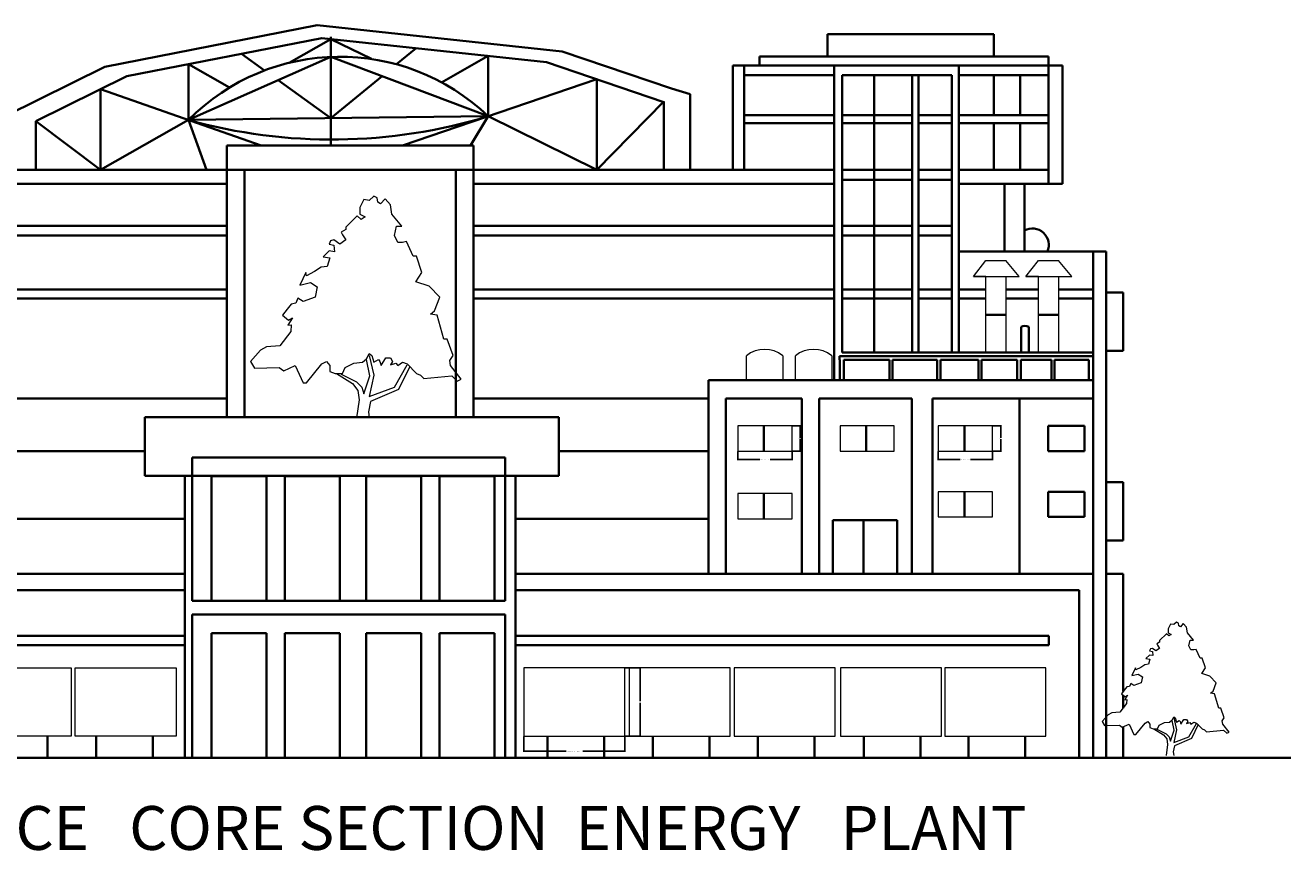
# Model space of a CAD drawing. Units: inches. Extents: x -362 to 223, y -437 to 70.
# Tile 2 of 5: x -124 to 180, y -437 to -239. Entities that reach past the tile are written whole.
import ezdxf

# ---------------------------------------------------------------- set-up
doc = ezdxf.new("R2010")
doc.units = ezdxf.units.IN
doc.header["$MEASUREMENT"] = 0
for name, color, linetype, lineweight in [('A-ANNO-DIMS', 2, 'Continuous', 18), ('A-ANNO-TEXT', 7, 'Continuous', 25), ('A-ELEV', 7, 'Continuous', 35), ('A-EQPM', 8, 'Continuous', 18), ('A-GLAZ', 4, 'Continuous', 18), ('L-PLNT', 3, 'Continuous', 13)]:
    doc.layers.add(name, color=color, linetype=linetype, lineweight=lineweight)
doc.styles.get("Standard").update_dxf_attribs({"font": 'arial.ttf'})
doc.dimstyles.get("Standard").update_dxf_attribs({"dimtxt": 0.18, "dimasz": 0.18, "dimexe": 0.18, "dimexo": 0.0625, "dimgap": 0.09, "dimtad": 0, "dimtih": 1, "dimtoh": 1, "dimdec": 4, "dimzin": 0, "dimdsep": 46, "dimtxsty": 'Standard', "dimcen": 0.09, "dimadec": 0, "dimazin": 0, "dimtfac": 1, "dimtdec": 4, "dimtofl": 0, "dimtmove": 0, "dimatfit": 3, "dimfxl": 1, "dimtolj": 1, "dimtzin": 0, "dimarcsym": 0})

# ---------------------------------------------------------------- blocks, each defined once
blk = doc.blocks.new('*U2')
for points in [[(22.0124, 137.721), (18.5475, 141.5624), (15.5282, 138.2446), (13.8028, 139.3505), (13.3714, 142.1153), (11.2148, 143.2214), (8.1954, 140.4564), (4.7447, 141.0094), (2.1567, 136.0326), (2.1567, 131.6088), (5.6074, 129.9499), (3.0193, 128.2909), (0.4313, 130.5029), (-6.9015, 123.3141), (-6.9015, 121.6552), (-9.9208, 119.9963), (-9.0581, 118.3373), (-6.9015, 115.0195), (-10.7835, 112.2546), (-14.6656, 115.0195), (-16.8222, 114.4665), (-17.6849, 112.2546), (-14.6656, 111.7016), (-14.2342, 107.2778), (-17.6065, 107.8307), (-21.5669, 103.9599), (-17.2536, 103.4069), (-18.9789, 97.8771), (-22.8609, 97.3241), (-27.1743, 94.5593), (-32.3504, 91.7944), (-32.7817, 94.0063), (-36.6638, 85.7116), (-29.7624, 87.3705), (-25.449, 84.6056), (-26.743, 77.9699), (-34.507, 75.205), (-37.9578, 77.4169), (-39.2518, 74.099), (-42.2711, 73.5461), (-44.8592, 70.2282), (-47.8786, 66.3574), (-43.9965, 63.0395), (-41.4085, 64.6985), (-44.3346, 59.8898), (-42.2089, 60.1377), (-42.5159, 55.7849), (-49.6039, 46.4502), (-58.2307, 45.8972), (-62.1127, 43.6853), (-68.5828, 36.4966), (-65.9947, 32.0727), (-50.0352, 32.6257), (-47.0159, 30.4138), (-39.6831, 33.7317), (-34.507, 22.6721), (-32.3504, 22.6721), (-22.4296, 34.8376), (-19.4102, 36.4966), (-17.2536, 33.7317), (-17.2536, 29.8608), (-13.8028, 28.7549), (-9.0581, 28.7549), (-7.3328, 32.6257), (-1.7254, 35.3906), (3.8821, 35.9436), (6.4701, 38.1555), (6.9014, 38.7085), (8.1954, 41.4734), (9.9208, 40.3674), (11.2148, 35.9436), (14.2341, 37.6025), (15.0968, 36.4966), (15.9595, 33.7317), (18.9789, 38.7085), (21.9982, 38.7085), (23.2922, 36.4966), (21.9982, 34.2847), (25.4489, 35.3906), (26.743, 33.7317), (29.7623, 35.9436), (32.7817, 34.8376), (38.8204, 28.7549), (41.4084, 27.6489), (43.5651, 25.437), (61.6813, 27.0959), (65.132, 23.7781), (67.7201, 24.884), (60.8186, 33.7317), (60.3873, 37.0495), (62.544, 40.3674), (58.662, 50.874), (56.5053, 50.874), (52.1919, 66.3574), (47.8785, 66.9103), (50.4665, 69.1222), (53.9172, 77.9699), (47.0158, 85.1586), (38.3891, 87.9235), (42.2711, 94.0063)], [(42.2711, 94.0063), (38.8204, 104.5129), (36.6637, 104.5129), (32.3503, 113.9135), (29.7623, 113.3605), (26.743, 113.3605), (24.5862, 117.7844), (25.8802, 123.8671), (29.331, 123.8671), (22.8609, 131.6088), (21.9982, 137.6916)], [(-9.9208, 28.2019), (0, 23.2251), (3.4507, 19.9072), (4.7447, 15.4834), (8.6267, 27.0959), (6.4701, 37.6025)], [(34.5071, 33.1787), (27.1743, 18.2483), (9.0581, 10.5066), (7.7641, 3.8708), (8.1954, 0)], [(8.1954, 40.3674), (11.2148, 27.6489), (8.1954, 13.8245), (24.5862, 19.9072), (32.7817, 34.2847)], [(-12.9401, 28.7549), (-2.588, 22.1191), (0.8626, 17.6953), (1.7253, 11.6125), (0, 0)]]:
    blk.add_lwpolyline(points)
blk = doc.blocks.new('WIN-STOREFRONT')
for p, q in [((24.23, 16.39), (0, 16.39)), ((0, 16.39), (0, 0)), ((24.23, 0), (24.23, 16.39)), ((0, 0), (6.79, 0)), ((6.79, 0), (24.23, 0))]:
    blk.add_line(p, q)
blk = doc.blocks.new('ROOF-VENT')
for p, q in [((0, 18.24), (2.99, 22.1)), ((2.99, 22.1), (7.83, 22.1)), ((11.03, 18.24), (7.83, 22.1)), ((2.99, 18.24), (0, 18.24)), ((0, 18.24), (11.03, 18.24)), ((2.99, 0), (2.99, 18.24)), ((2.99, 18.24), (7.83, 18.24)), ((7.83, 18.24), (7.83, 0))]:
    blk.add_line(p, q)
blk = doc.blocks.new('WIN-C')
for p, q in [((13.02, 6.07), (0, 6.07)), ((0, 6.07), (0, 5.53)), ((0, 5.53), (0, 0)), ((13.02, 0), (13.02, 6.07)), ((0, 0), (13.02, 0))]:
    blk.add_line(p, q)
blk = doc.blocks.new('WIN-D')
for p, q in [((13.02, 6.07), (0, 6.07)), ((0, 6.07), (0, 5.53)), ((0, 5.53), (0, 0)), ((13.02, 6.07), (11.9, 6.07)), ((13.02, 0), (13.02, 6.07)), ((0, 0), (13.02, 0)), ((11.9, 0), (13.02, 0))]:
    blk.add_line(p, q)
blk = doc.blocks.new('ROOF-DOME')
for p, q in [((0, 0), (0, 5.87)), ((8.74, 5.87), (8.74, 0))]:
    blk.add_line(p, q)
blk.add_arc((4.37, 0.37), 7.03, 51.5309, 128.4691)
blk = doc.blocks.new('*D17')
at = {"layer": 'A-ANNO-DIMS', "color": 0, "lineweight": -2, "transparency": 16777216}
for p, q in [((-4.56, -409.76), (-4.56, -413.51)), ((19.67, -409.76), (19.67, -413.51)), ((-4.38, -413.33), (5.54, -413.33)), ((19.49, -413.33), (9.57, -413.33))]:
    blk.add_line(p, q, dxfattribs=at)
at = {"layer": 'A-ANNO-DIMS', "color": 0, "transparency": 16777216}
for points in [[(-4.38, -413.3), (-4.38, -413.36), (-4.56, -413.33)], [(19.49, -413.3), (19.49, -413.36), (19.67, -413.33)]]:
    blk.add_solid(points, dxfattribs=at)
at = {"layer": 'Defpoints', "color": 0, "transparency": 16777216}
for p in [(-4.56, -409.69), (19.67, -409.69), (19.67, -413.33)]:
    blk.add_point(p, dxfattribs=at)
at = {"layer": 'A-ANNO-DIMS', "color": 0, "transparency": 16777216, "insert": (7.56, -413.33), "char_height": 0.18, "attachment_point": 5}
blk.add_mtext('\\A1;STOREFRONT WINDOW 24 TYP.', dxfattribs=at)
blk = doc.blocks.new('*D18')
at = {"layer": 'A-ANNO-DIMS', "color": 0, "lineweight": -2, "transparency": 16777216}
for p, q in [((19.73, -393.31), (23.48, -393.31)), ((23.3, -393.49), (23.3, -401.32)), ((23.3, -409.51), (23.3, -401.68)), ((19.73, -409.69), (23.48, -409.69))]:
    blk.add_line(p, q, dxfattribs=at)
at = {"layer": 'A-ANNO-DIMS', "color": 0, "transparency": 16777216}
for points in [[(23.27, -393.49), (23.33, -393.49), (23.3, -393.31)], [(23.27, -409.51), (23.33, -409.51), (23.3, -409.69)]]:
    blk.add_solid(points, dxfattribs=at)
at = {"layer": 'Defpoints', "color": 0, "transparency": 16777216}
for p in [(19.67, -393.31), (23.3, -393.31), (19.67, -409.69)]:
    blk.add_point(p, dxfattribs=at)
at = {"layer": 'A-ANNO-DIMS', "color": 0, "transparency": 16777216, "insert": (23.3, -401.5), "char_height": 0.18, "attachment_point": 5}
blk.add_mtext('\\A1;16 TYP.', dxfattribs=at)
blk = doc.blocks.new('*D25')
at = {"layer": 'A-ANNO-DIMS', "color": 0, "lineweight": -2, "transparency": 16777216}
for p, q in [((46.79, -341.37), (46.79, -343.44)), ((46.97, -343.26), (52.05, -343.26)), ((59.62, -343.26), (54.54, -343.26)), ((59.8, -341.37), (59.8, -343.44))]:
    blk.add_line(p, q, dxfattribs=at)
at = {"layer": 'A-ANNO-DIMS', "color": 0, "transparency": 16777216}
for points in [[(46.97, -343.23), (46.97, -343.29), (46.79, -343.26)], [(59.62, -343.23), (59.62, -343.29), (59.8, -343.26)]]:
    blk.add_solid(points, dxfattribs=at)
at = {"layer": 'Defpoints', "color": 0, "transparency": 16777216}
for p in [(46.79, -341.31), (59.8, -341.31), (59.8, -343.26)]:
    blk.add_point(p, dxfattribs=at)
at = {"layer": 'A-ANNO-DIMS', "color": 0, "transparency": 16777216, "insert": (53.29, -343.26), "char_height": 0.18, "attachment_point": 5}
blk.add_mtext('\\A1;WINDOW C 13 TYP.', dxfattribs=at)
blk = doc.blocks.new('*D26')
at = {"layer": 'A-ANNO-DIMS', "color": 0, "lineweight": -2, "transparency": 16777216}
for p, q in [((59.86, -335.24), (61.93, -335.24)), ((61.75, -335.42), (61.75, -338.09)), ((61.75, -341.13), (61.75, -338.45)), ((59.86, -341.31), (61.93, -341.31))]:
    blk.add_line(p, q, dxfattribs=at)
at = {"layer": 'A-ANNO-DIMS', "color": 0, "transparency": 16777216}
for points in [[(61.72, -335.42), (61.78, -335.42), (61.75, -335.24)], [(61.72, -341.13), (61.78, -341.13), (61.75, -341.31)]]:
    blk.add_solid(points, dxfattribs=at)
at = {"layer": 'Defpoints', "color": 0, "transparency": 16777216}
for p in [(59.8, -335.24), (61.75, -335.24), (59.8, -341.31)]:
    blk.add_point(p, dxfattribs=at)
at = {"layer": 'A-ANNO-DIMS', "color": 0, "transparency": 16777216, "insert": (61.75, -338.27), "char_height": 0.18, "attachment_point": 5}
blk.add_mtext('\\A1;6 TYP.', dxfattribs=at)
blk = doc.blocks.new('*D29')
at = {"layer": 'A-ANNO-DIMS', "color": 0, "lineweight": -2, "transparency": 16777216}
for p, q in [((94.91, -341.37), (94.91, -343.44)), ((95.09, -343.26), (100.18, -343.26)), ((107.75, -343.26), (102.66, -343.26)), ((107.93, -341.37), (107.93, -343.44))]:
    blk.add_line(p, q, dxfattribs=at)
at = {"layer": 'A-ANNO-DIMS', "color": 0, "transparency": 16777216}
for points in [[(95.09, -343.23), (95.09, -343.29), (94.91, -343.26)], [(107.75, -343.23), (107.75, -343.29), (107.93, -343.26)]]:
    blk.add_solid(points, dxfattribs=at)
at = {"layer": 'Defpoints', "color": 0, "transparency": 16777216}
for p in [(94.91, -341.31), (107.93, -341.31), (107.93, -343.26)]:
    blk.add_point(p, dxfattribs=at)
at = {"layer": 'A-ANNO-DIMS', "color": 0, "transparency": 16777216, "insert": (101.42, -343.26), "char_height": 0.18, "attachment_point": 5}
blk.add_mtext('\\A1;WINDOW D 13 TYP.', dxfattribs=at)
blk = doc.blocks.new('*D30')
at = {"layer": 'A-ANNO-DIMS', "color": 0, "lineweight": -2, "transparency": 16777216}
for p, q in [((107.99, -335.24), (110.06, -335.24)), ((109.88, -335.42), (109.88, -338.09)), ((109.88, -341.13), (109.88, -338.45)), ((107.99, -341.31), (110.06, -341.31))]:
    blk.add_line(p, q, dxfattribs=at)
at = {"layer": 'A-ANNO-DIMS', "color": 0, "transparency": 16777216}
for points in [[(109.85, -335.42), (109.91, -335.42), (109.88, -335.24)], [(109.85, -341.13), (109.91, -341.13), (109.88, -341.31)]]:
    blk.add_solid(points, dxfattribs=at)
at = {"layer": 'Defpoints', "color": 0, "transparency": 16777216}
for p in [(107.93, -335.24), (109.88, -335.24), (107.93, -341.31)]:
    blk.add_point(p, dxfattribs=at)
at = {"layer": 'A-ANNO-DIMS', "color": 0, "transparency": 16777216, "insert": (109.88, -338.27), "char_height": 0.18, "attachment_point": 5}
blk.add_mtext('\\A1;6 TYP.', dxfattribs=at)

msp = doc.modelspace()

# ---------------------------------------------------------------- linework, layer by layer
at = {"layer": 'A-ELEV'}
for p, q in [((-105.16, -249.03), (-54.21, -239.06)), ((-54.21, -239.06), (4.61, -245.36)), ((-99.88, -251.28), (-53.13, -242.13)), ((-50.9, -242.37), (-60.97, -248.08)), ((-53.13, -242.13), (0.84, -247.91)), ((-50.9, -241.82), (-50.9, -267.9)), ((-41.18, -247.15), (-50.9, -242.37)), ((68.27, -246.58), (68.27, -241.22)), ((68.27, -241.22), (108.22, -241.22)), ((108.22, -241.22), (108.22, -246.58)), ((-66.82, -249.9), (-72.38, -245.89)), ((-35.15, -248.42), (-30.45, -244.56)), ((4.61, -245.36), (30.87, -254.27)), ((-128.95, -260.83), (-105.16, -249.03)), ((-85.13, -261.78), (-50.9, -246.64)), ((-85.13, -261.78), (-85.13, -248.39)), ((-75.27, -254.01), (-85.13, -248.39)), ((-50.9, -246.64), (-13.18, -260.91)), ((-24.33, -252.76), (-13.18, -246.41)), ((-13.18, -260.91), (-13.18, -246.41)), ((0.84, -247.91), (29.02, -257.48)), ((51.95, -248.69), (45.6, -248.69)), ((45.6, -248.69), (45.6, -273.74)), ((48.33, -273.74), (48.33, -248.69)), ((121.39, -246.58), (51.95, -246.58)), ((51.95, -246.58), (51.95, -248.69)), ((51.95, -248.69), (121.39, -248.69)), ((69.89, -248.72), (69.89, -317.63)), ((99.85, -248.69), (99.85, -317.63)), ((121.39, -277.1), (121.39, -246.58)), ((121.39, -248.69), (124.7, -248.69)), ((124.7, -248.69), (124.7, -273.74)), ((-121.72, -262.11), (-99.88, -251.28)), ((-50.9, -261.37), (-38.63, -251.28)), ((-33.73, -267.9), (12.95, -252.02)), ((12.95, -273.74), (12.95, -252.02)), ((48.33, -251.06), (69.89, -251.06)), ((72.44, -251.06), (71.85, -251.06)), ((71.85, -251.06), (71.85, -317.63)), ((71.85, -251.06), (88.65, -251.06)), ((72.44, -251.06), (98.13, -251.06)), ((79.54, -251.06), (79.54, -317.63)), ((88.65, -251.06), (88.65, -317.63)), ((90.12, -251.06), (90.12, -317.63)), ((90.12, -251.06), (98.13, -251.06)), ((98.13, -251.06), (98.13, -317.63)), ((99.85, -251.06), (121.39, -251.06)), ((108.22, -251.06), (108.22, -260.65)), ((114.59, -251.06), (114.59, -260.65)), ((-106.21, -273.74), (-106.21, -254.41)), ((-67.62, -267.9), (-106.21, -254.41)), ((-50.9, -261.37), (-63.57, -252.24)), ((30.87, -254.27), (35.32, -255.62)), ((12.95, -273.74), (29.02, -257.32)), ((29.02, -257.32), (29.02, -273.74)), ((35.32, -255.62), (35.32, -273.74)), ((-85.13, -261.78), (-13.18, -260.91)), ((-13.18, -260.91), (-85.13, -261.78)), ((-13.18, -260.91), (-17.39, -267.9)), ((12.95, -273.74), (-13.18, -260.91)), ((48.33, -260.65), (69.89, -260.65)), ((71.85, -260.65), (88.65, -260.65)), ((90.12, -260.65), (98.13, -260.65)), ((99.85, -260.65), (121.39, -260.65)), ((-121.72, -273.95), (-121.72, -262.11)), ((-106.21, -273.74), (-121.72, -262.11)), ((-85.13, -261.78), (-106.21, -273.74)), ((-85.13, -261.78), (-80.8, -273.74)), ((48.33, -262.59), (69.89, -262.59)), ((71.85, -262.59), (88.65, -262.59)), ((90.12, -262.59), (98.13, -262.59)), ((99.85, -262.59), (121.39, -262.59)), ((108.22, -262.59), (108.22, -273.74)), ((114.59, -262.59), (114.59, -273.74)), ((-75.93, -273.74), (-75.93, -267.9)), ((-75.93, -267.9), (-16.66, -267.9)), ((-16.66, -267.9), (-16.66, -273.74)), ((-138.19, -273.74), (-97.81, -273.74)), ((-106.21, -273.74), (-106.21, -273.74)), ((-97.81, -273.74), (-75.93, -273.74)), ((-75.93, -273.74), (-75.93, -333.13)), ((-71.68, -273.74), (-75.93, -273.74)), ((-75.93, -273.74), (-50.9, -273.74)), ((-71.68, -276.11), (-71.68, -273.74)), ((-71.68, -273.74), (-20.92, -273.74)), ((-71.68, -333.13), (-71.68, -276.11)), ((-20.92, -276.11), (-20.92, -273.74)), ((-20.92, -273.74), (-16.66, -273.74)), ((-20.92, -333.13), (-20.92, -276.11)), ((5.21, -273.74), (-16.66, -273.74)), ((-16.66, -273.74), (-16.66, -333.13)), ((45.6, -273.74), (5.21, -273.74)), ((45.6, -273.74), (48.33, -273.74)), ((48.33, -273.74), (69.89, -273.74)), ((71.85, -273.74), (88.65, -273.74)), ((71.85, -276.18), (88.65, -276.18)), ((90.12, -273.74), (98.13, -273.74)), ((90.12, -276.18), (98.13, -276.18)), ((99.85, -273.74), (121.39, -273.74)), ((124.7, -273.74), (124.7, -277.1)), ((-162.48, -277.1), (-105.45, -277.1)), ((-105.45, -277.1), (-75.93, -277.1)), ((12.86, -277.1), (-16.66, -277.1)), ((69.89, -277.1), (12.86, -277.1)), ((48.33, -277.1), (69.89, -277.1)), ((121.39, -277.1), (99.85, -277.1)), ((99.85, -277.1), (121.39, -277.1)), ((110.79, -277.1), (110.79, -288.32)), ((115.56, -277.1), (115.56, -288.32)), ((124.7, -277.1), (121.39, -277.1)), ((71.85, -287.17), (88.65, -287.17)), ((90.12, -287.17), (98.13, -287.17)), ((110.79, -288.32), (110.79, -293.39)), ((115.56, -288.32), (115.56, -293.39)), ((-162.48, -289.53), (-75.93, -289.53)), ((69.89, -289.53), (-16.66, -289.53)), ((71.85, -289.53), (88.65, -289.53)), ((90.12, -289.53), (98.13, -289.53)), ((110.79, -293.39), (99.85, -293.39)), ((110.79, -293.39), (132.09, -293.39)), ((132.09, -293.39), (132.09, -338.07)), ((132.09, -293.39), (135.24, -293.39)), ((135.24, -293.39), (135.24, -370.73)), ((-162.48, -302.45), (-75.93, -302.45)), ((69.89, -302.45), (-16.66, -302.45)), ((71.85, -302.45), (88.65, -302.45)), ((90.12, -302.45), (98.13, -302.45)), ((99.85, -302.45), (106.31, -302.45)), ((111.15, -302.45), (118.92, -302.45)), ((123.77, -302.45), (132.09, -302.45)), ((135.24, -303.22), (139.26, -303.22)), ((139.26, -303.22), (139.26, -313.58)), ((-162.48, -304.65), (-75.93, -304.65)), ((69.89, -304.65), (-16.66, -304.65)), ((71.85, -304.65), (88.65, -304.65)), ((90.12, -304.65), (98.13, -304.65)), ((99.85, -304.65), (106.31, -304.65)), ((111.15, -304.65), (118.92, -304.65)), ((123.77, -304.65), (132.09, -304.65)), ((106.31, -308.56), (111.15, -308.56)), ((118.92, -308.56), (123.77, -308.56)), ((114.79, -317.63), (114.79, -311.48)), ((114.79, -311.48), (114.79, -311.48)), ((116.63, -311.48), (116.63, -317.63)), ((139.26, -313.58), (139.26, -317.17)), ((69.89, -317.63), (69.89, -324.26)), ((71.21, -319.37), (71.21, -318.52)), ((71.21, -318.52), (132.09, -318.52)), ((132.09, -317.63), (71.85, -317.63)), ((139.26, -317.17), (135.24, -317.17)), ((71.24, -324.26), (71.24, -319.37)), ((72.2, -319.37), (83.15, -319.37)), ((72.2, -324.26), (72.2, -319.37)), ((83.15, -324.26), (83.15, -319.37)), ((83.88, -324.26), (83.88, -319.37)), ((83.88, -319.37), (94.62, -319.37)), ((94.62, -324.26), (94.62, -319.37)), ((95.4, -324.26), (95.4, -319.37)), ((95.4, -319.37), (104.52, -319.37)), ((104.52, -324.26), (104.52, -319.37)), ((105.31, -324.26), (105.31, -319.37)), ((105.31, -319.37), (113.82, -319.37)), ((113.82, -324.26), (113.82, -319.37)), ((114.71, -324.26), (114.71, -319.37)), ((114.71, -319.37), (122.06, -319.37)), ((122.06, -324.26), (122.06, -319.37)), ((122.84, -324.26), (122.84, -319.37)), ((122.84, -319.37), (131.08, -319.37)), ((131.08, -324.26), (131.08, -319.37)), ((39.77, -370.73), (39.77, -324.26)), ((39.77, -324.26), (132.09, -324.26)), ((-132.36, -328.62), (-75.93, -328.62)), ((39.77, -328.62), (-16.66, -328.62)), ((43.86, -370.73), (43.86, -328.62)), ((43.86, -328.62), (62.15, -328.62)), ((62.15, -328.62), (62.15, -370.73)), ((66.27, -328.62), (66.27, -370.73)), ((66.27, -328.62), (88.53, -328.62)), ((88.53, -328.62), (88.53, -370.73)), ((93.48, -328.62), (93.48, -370.73)), ((93.48, -328.62), (132.09, -328.62)), ((114.36, -328.62), (114.36, -370.73)), ((-95.58, -347.18), (-95.58, -333.13)), ((-95.58, -333.13), (3.82, -333.13)), ((3.82, -333.13), (3.82, -347.18)), ((53.03, -335.24), (53.03, -341.31)), ((77.57, -335.24), (77.57, -341.31)), ((101.16, -335.24), (101.16, -341.31)), ((129.99, -335.24), (121.25, -335.24)), ((121.25, -335.24), (121.25, -341.31)), ((129.99, -341.31), (129.99, -335.24)), ((132.09, -338.07), (132.09, -370.73)), ((-132.36, -341.31), (-95.58, -341.31)), ((-84.21, -377.23), (-84.21, -342.82)), ((-84.21, -342.82), (-9.05, -342.82)), ((-9.05, -342.82), (-9.05, -377.23)), ((39.77, -341.31), (3.82, -341.31)), ((121.25, -341.31), (129.99, -341.31)), ((-85.99, -347.18), (-95.58, -347.18)), ((-85.99, -385.66), (-85.99, -347.18)), ((-85.99, -347.18), (-6.6, -347.18)), ((-79.57, -377.23), (-79.57, -347.32)), ((-79.57, -347.32), (-66.36, -347.32)), ((-66.36, -347.32), (-66.36, -377.23)), ((-62, -377.23), (-62, -347.32)), ((-62, -347.32), (-48.79, -347.32)), ((-48.79, -347.32), (-48.79, -377.23)), ((-42.42, -377.23), (-42.42, -347.32)), ((-42.42, -347.32), (-29.21, -347.32)), ((-29.21, -347.32), (-29.21, -377.23)), ((-24.85, -377.23), (-24.85, -347.32)), ((-24.85, -347.32), (-11.64, -347.32)), ((-11.64, -347.32), (-11.64, -377.23)), ((-6.6, -347.18), (-6.6, -385.66)), ((3.82, -347.18), (-6.6, -347.18)), ((135.24, -348.77), (139.26, -348.77)), ((139.26, -348.77), (139.26, -359.13)), ((53.03, -351.45), (53.03, -357.51)), ((101.16, -351.02), (101.16, -357.09)), ((129.99, -351.02), (121.25, -351.02)), ((121.25, -351.02), (121.25, -357.09)), ((129.99, -357.09), (129.99, -351.02)), ((-132.36, -357.51), (-85.99, -357.51)), ((39.77, -357.51), (-6.6, -357.51)), ((69.57, -370.73), (69.57, -357.88)), ((69.57, -357.88), (85, -357.88)), ((76.93, -370.73), (76.93, -357.88)), ((85, -357.88), (85, -370.73)), ((121.25, -357.09), (129.99, -357.09)), ((139.26, -359.13), (139.26, -362.71)), ((139.26, -362.71), (135.24, -362.71)), ((-224.68, -370.73), (-85.99, -370.73)), ((132.09, -370.73), (-6.6, -370.73)), ((132.09, -370.73), (132.09, -414.88)), ((135.24, -370.73), (139.25, -370.73)), ((135.24, -370.73), (135.24, -414.88)), ((139.25, -370.73), (139.25, -399.03)), ((-221.28, -374.68), (-85.99, -374.68)), ((128.69, -374.68), (-6.6, -374.68)), ((128.69, -414.88), (128.69, -374.68)), ((-67.23, -377.23), (-84.21, -377.23)), ((-9.05, -377.23), (-79.57, -377.23)), ((-49.65, -377.23), (-66.36, -377.23)), ((-30.08, -377.23), (-48.79, -377.23)), ((-25.37, -377.23), (-16.66, -377.23)), ((-84.21, -414.88), (-84.21, -380.47)), ((-84.21, -380.47), (-9.05, -380.47)), ((-9.05, -380.47), (-9.05, -414.88)), ((-85.99, -385.66), (-214.01, -385.66)), ((-85.99, -409.69), (-85.99, -385.66)), ((-79.57, -414.88), (-79.57, -384.97)), ((-79.57, -384.97), (-66.36, -384.97)), ((-66.36, -384.97), (-66.36, -414.88)), ((-62, -414.88), (-62, -384.97)), ((-62, -384.97), (-48.79, -384.97)), ((-48.79, -384.97), (-48.79, -414.88)), ((-42.42, -414.88), (-42.42, -384.97)), ((-42.42, -384.97), (-29.21, -384.97)), ((-29.21, -384.97), (-29.21, -414.88)), ((-24.85, -414.88), (-24.85, -384.97)), ((-24.85, -384.97), (-11.64, -384.97)), ((-11.64, -384.97), (-11.64, -414.88)), ((-6.6, -409.69), (-6.6, -385.66)), ((-6.6, -385.66), (121.42, -385.66)), ((121.42, -385.66), (121.42, -387.9)), ((-85.99, -387.9), (-214.01, -387.9)), ((-6.6, -387.9), (121.42, -387.9)), ((139.25, -399.84), (139.25, -402.96)), ((-118.94, -414.77), (-118.94, -409.69)), ((-107.26, -414.77), (-107.26, -409.69)), ((-93.68, -414.77), (-93.68, -409.69)), ((-85.99, -409.69), (-85.99, -414.88)), ((-6.6, -409.69), (-6.6, -414.88)), ((1.08, -414.77), (1.08, -409.69)), ((14.67, -414.77), (14.67, -409.69)), ((26.35, -414.77), (26.35, -409.69)), ((39.94, -414.77), (39.94, -409.69)), ((51.56, -414.77), (51.56, -409.69)), ((65.15, -414.77), (65.15, -409.69)), ((77.06, -414.77), (77.06, -409.69)), ((90.65, -414.77), (90.65, -409.69)), ((102.13, -414.77), (102.13, -409.69)), ((115.72, -414.77), (115.72, -409.69)), ((139.25, -407.47), (139.25, -414.88)), ((-224.68, -414.88), (-75.93, -414.88)), ((-25.37, -414.88), (-130.92, -414.88)), ((-67.23, -414.88), (-75.93, -414.88)), ((-49.65, -414.88), (-58.36, -414.88)), ((-30.08, -414.88), (-38.78, -414.88)), ((-25.37, -414.88), (-16.66, -414.88)), ((-12.51, -414.88), (-21.21, -414.88)), ((132.09, -414.88), (-16.66, -414.88)), ((139.25, -414.88), (132.09, -414.88)), ((135.24, -414.88), (179.5, -414.88))]:
    msp.add_line(p, q, dxfattribs=at)
for points in [[(-162.48, -287.17), (-75.93, -287.17)], [(69.89, -287.17), (-16.66, -287.17)]]:
    msp.add_lwpolyline(points, dxfattribs=at)
for centre, radius, start, end in [((-48.71, -297.84), 51.25, 46.1074, 135.2891), ((-50.66, -137.81), 128.68, 254.4622, 286.9343), ((117.46, -291.82), 3.98, 336.8313, 118.5268), ((115.71, -312.87), 1.66, 56.4994, 123.5006)]:
    msp.add_arc(centre, radius, start, end, dxfattribs=at)

# ---------------------------------------------------------------- block references
at = {"layer": 'A-EQPM'}
for name, p in [('ROOF-VENT', (103.32, -317.63)), ('ROOF-VENT', (115.94, -317.63)), ('ROOF-DOME', (48.83, -324.25)), ('ROOF-DOME', (60.6, -324.25))]:
    msp.add_blockref(name, p, dxfattribs=at)
at = {"layer": 'A-GLAZ'}
for name, p in [('WIN-C', (46.78, -341.31)), ('WIN-C', (71.32, -341.31)), ('WIN-D', (94.91, -341.31)), ('WIN-C', (46.78, -357.51)), ('WIN-D', (94.91, -357.09)), ('WIN-STOREFRONT', (-4.56, -409.69)), ('WIN-STOREFRONT', (20.71, -409.69)), ('WIN-STOREFRONT', (45.92, -409.69)), ('WIN-STOREFRONT', (71.42, -409.69)), ('WIN-STOREFRONT', (96.49, -409.69))]:
    msp.add_blockref(name, p, dxfattribs=at)
at = {"layer": 'A-GLAZ', "extrusion": (0, 0, -1), "zscale": -1}
for p in [(113.3, -409.69), (88.04, -409.69)]:
    msp.add_blockref('WIN-STOREFRONT', p, dxfattribs=at)
at = {"layer": 'L-PLNT'}
for p, xscale, yscale, zscale in [((-44.77, -333.29), 0.3714056564467734, 0.3714056564467734, 0.3714056564467734), ((149.58, -414.35), 0.2236213924327499, 0.2236213924327499, 0.2236213924327499)]:
    msp.add_blockref('*U2', p, dxfattribs=dict(at, xscale=xscale, yscale=yscale, zscale=zscale))

# ---------------------------------------------------------------- texts
at = {"layer": 'A-ANNO-TEXT'}
msp.add_text('MECHANICAL  SERVICE   CORE SECTION  ENERGY   PLANT ', height=10.5337, dxfattribs=at).set_placement((-260.49, -437.02))

# ---------------------------------------------------------------- dimensions: what is measured, and where the dimension line sits
at = {"layer": 'A-ANNO-DIMS'}
for base, p1, p2, picture, middle in [((61.75, -335.24), (59.8, -341.31), (59.8, -335.24), '*D26', (61.75, -338.27)), ((109.88, -335.24), (107.93, -341.31), (107.93, -335.24), '*D30', (109.88, -338.27)), ((23.3, -393.31), (19.67, -409.69), (19.67, -393.31), '*D18', (23.3, -401.5))]:
    dim = msp.add_linear_dim(base=base, p1=p1, p2=p2, angle=90, text='<> TYP.', dimstyle='Standard', override={"dimdec": 0, "dimlfac": 1, "dimrnd": 0, "dimzin": 0, "dimdsep": 46, "dimlunit": 2}, dxfattribs=at)
    dim.commit()
    dim.dimension.update_dxf_attribs({"geometry": picture, "text_midpoint": middle})
for base, p1, p2, text, picture, middle in [((59.8, -343.26), (46.79, -341.31), (59.8, -341.31), 'WINDOW C <> TYP.', '*D25', (53.29, -343.26)), ((107.93, -343.26), (94.91, -341.31), (107.93, -341.31), 'WINDOW D <> TYP.', '*D29', (101.42, -343.26)), ((19.67, -413.33), (-4.56, -409.69), (19.67, -409.69), 'STOREFRONT WINDOW <> TYP.', '*D17', (7.56, -413.33))]:
    dim = msp.add_linear_dim(base=base, p1=p1, p2=p2, text=text, dimstyle='Standard', override={"dimdec": 0, "dimlfac": 1, "dimrnd": 0, "dimzin": 0, "dimdsep": 46, "dimlunit": 2}, dxfattribs=at)
    dim.commit()
    dim.dimension.update_dxf_attribs({"geometry": picture, "text_midpoint": middle})

doc.saveas('drawing.dxf')
